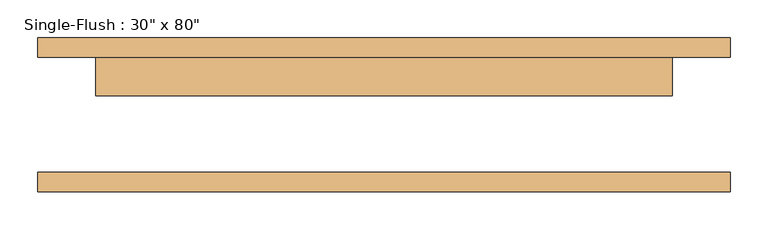
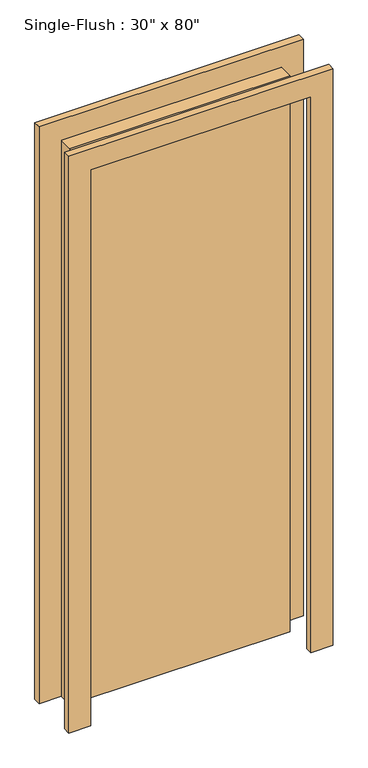
"""IFC4 building model written with IfcOpenShell, lengths in millimetres: door geometry."""

from ifc_helpers import new_model, si_unit, frame, origin, origin_with_axes, place, context, project, spatial, polyline, outline, extrude, source, transform, mapped, element, save


def door_059fdd7e(model_context):
    return source(origin(), model_context, "Body", "SweptSolid", [
        extrude(outline(polyline([(2108.2, -457.2), (0.0, -457.2), (0.0, -381.0), (2032.0, -381.0), (2032.0, 381.0), (0.0, 381.0), (0.0, 457.2), (2108.2, 457.2), (2108.2, -457.2)])), frame((0.0, 76.2, 0.0), z_axis=(0.0, 1.0, 0.0), x_axis=(0.0, 0.0, 1.0)), (0.0, 0.0, 1.0), 25.4),
        extrude(outline(polyline([(2108.2, 457.2), (2108.2, -457.2), (0.0, -457.2), (0.0, -381.0), (2032.0, -381.0), (2032.0, 381.0), (0.0, 381.0), (0.0, 457.2), (2108.2, 457.2)])), frame((0.0, -101.6, 0.0), z_axis=(0.0, 1.0, 0.0), x_axis=(0.0, 0.0, 1.0)), (0.0, 0.0, 1.0), 25.4),
        extrude(outline(polyline([(381.0, 25.4), (-381.0, 25.4), (-381.0, 76.2), (381.0, 76.2), (381.0, 25.4)])), origin_with_axes(), (0.0, 0.0, 1.0), 2032.0),
    ])


if __name__ == "__main__":
    model = new_model("IFC4")
    model_context = context("Model", 3, world=origin())
    ifc_project = project(units=[si_unit("LENGTHUNIT", "METRE", prefix="MILLI")], contexts=[model_context])
    site = spatial("IfcSite", under=ifc_project)
    building = spatial("IfcBuilding", under=site)
    placement = place(None, origin())
    door_shape = door_059fdd7e(model_context)
    element("IfcDoor", 1, ObjectType="Single-Flush : 30\" x 80\"", at=placement, inside=building, context=model_context, shape_type="MappedRepresentation", body=[
        mapped(door_shape, transform((0.0, 0.0, 0.0), x_axis=(1.0, 0.0, 0.0), y_axis=(0.0, 1.0, 0.0), z_axis=(0.0, 0.0, 1.0))),
    ])
    save(model, "model.ifc")

# Revit data of these elements
# Type "Single-Flush : 30\" x 80\""
#   Type Mark = "5"
#   Construction Type Id = "MDOOR"
#   Assembly Code = "C1020"
#   Analytic Construction = "Metal"
#   Thickness = 0' - 2"
#   Heat Transfer Coefficient (U) = 0.651978 BTU/(h·ft²·°F)
#   Height = 6' - 8"
#   Trim Projection Ext = 0' - 1"
#   Trim Projection Int = 0' - 1"
#   Trim Width = 0' - 3"
#   Width = 2' - 6"
#   Define Thermal Properties by = 1
#   Door Material = Door - Panel
#   Frame Material = Door - Frame
#   Visual Light Transmittance = 0
#   Solar Heat Gain Coefficient = 0
#   Function = (empty or 0)
#   Wall Closure = (empty or 0)
# Element 1 (IfcDoor, "Single-Flush : 30\" x 80\"")
#   Materials on its faces: "Door - Frame", "Door - Panel"
# Materials
#   "Door - Panel": class "Wood", colour RGB 210 159 95, transparency 0
#   "Door - Frame": colour RGB 118 70 51, transparency 0
